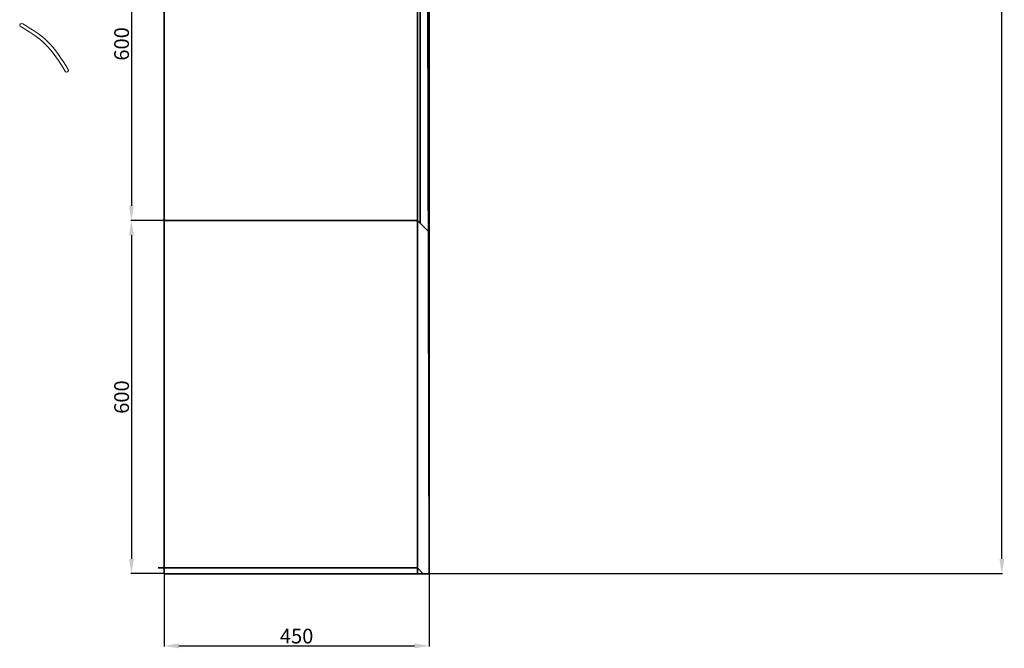
# Model space of a CAD drawing. Units: millimetres. Extents: x 11557 to 15272, y 8572 to 13242.
# Tile 2 of 4: x 13600 to 15272, y 8572 to 9640. Entities that reach past the tile are written whole.
import ezdxf

# ---------------------------------------------------------------- set-up
doc = ezdxf.new("R2010")
doc.units = ezdxf.units.MM
for name, color, linetype, lineweight in [('A-ANNO-DIMS', 2, 'Continuous', 18), ('A-FURN-BASE', 7, 'Continuous', 35), ('A-FURN-HARD', 8, 'Continuous', 18)]:
    doc.layers.add(name, color=color, linetype=linetype, lineweight=lineweight)
doc.styles.get("Standard").update_dxf_attribs({"font": 'arial.ttf'})
doc.dimstyles.new('ISO-25', dxfattribs={"dimtxt": 25, "dimasz": 25, "dimexe": 1.25, "dimexo": 0.625, "dimtad": 1, "dimdec": 1, "dimtxsty": 'Standard', "dimcen": 2.5, "dimadec": 0, "dimazin": 0, "dimtfac": 1, "dimtdec": 1, "dimtmove": 0, "dimatfit": 3, "dimfxl": 1, "dimarcsym": 0})

# ---------------------------------------------------------------- blocks, each defined once
blk = doc.blocks.new('*D1')
at = {"layer": 'A-ANNO-DIMS', "color": 0, "lineweight": -2, "transparency": 16777216}
for p, q in [((13844.6, 9298.9), (13788.4, 9298.9)), ((13789.6, 9273.9), (13789.6, 8723.9)), ((13844.6, 8698.9), (13788.4, 8698.9))]:
    blk.add_line(p, q, dxfattribs=at)
at = {"layer": 'A-ANNO-DIMS', "color": 0, "transparency": 16777216}
for points in [[(13785.5, 9273.9), (13793.8, 9273.9), (13789.6, 9298.9)], [(13785.5, 8723.9), (13793.8, 8723.9), (13789.6, 8698.9)]]:
    blk.add_solid(points, dxfattribs=at)
at = {"layer": 'Defpoints', "color": 0, "transparency": 16777216}
for p in [(13845.2, 9298.9, 720), (13789.6, 8698.9), (13845.2, 8698.9, 720)]:
    blk.add_point(p, dxfattribs=at)
at = {"layer": 'A-ANNO-DIMS', "color": 0, "transparency": 16777216, "insert": (13776.2, 8998.9), "char_height": 25, "attachment_point": 5, "rotation": 90}
blk.add_mtext('600', dxfattribs=at)
blk = doc.blocks.new('*D2')
at = {"layer": 'A-ANNO-DIMS', "color": 0, "lineweight": -2, "transparency": 16777216}
for p, q in [((13844.6, 9898.9), (13788.4, 9898.9)), ((13789.6, 9873.9), (13789.6, 9323.9)), ((13844.6, 9298.9), (13788.4, 9298.9))]:
    blk.add_line(p, q, dxfattribs=at)
at = {"layer": 'A-ANNO-DIMS', "color": 0, "transparency": 16777216}
for points in [[(13785.5, 9873.9), (13793.8, 9873.9), (13789.6, 9898.9)], [(13785.5, 9323.9), (13793.8, 9323.9), (13789.6, 9298.9)]]:
    blk.add_solid(points, dxfattribs=at)
at = {"layer": 'Defpoints', "color": 0, "transparency": 16777216}
for p in [(13845.2, 9898.9, 720), (13789.6, 9298.9), (13845.2, 9298.9, 720)]:
    blk.add_point(p, dxfattribs=at)
at = {"layer": 'A-ANNO-DIMS', "color": 0, "transparency": 16777216, "insert": (13776.2, 9598.9), "char_height": 25, "attachment_point": 5, "rotation": 90}
blk.add_mtext('600', dxfattribs=at)
blk = doc.blocks.new('BASE-CABINET-PULL')
for centre, radius, start, end in [((3, 79.7, -122.8), 3.04, 50.0455, 215.1607), ((79.2, 3.1, -122.8), 3.13, 238.0113, 27.1949)]:
    blk.add_arc(centre, radius, start, end)
for points in [[(77.6, 0.5, -122.8), (66.9, 17.8, -122.8), (47.2, 49.7, -122.8), (15.2, 69.1, -122.8), (0.5, 77.9, -122.8)], [(82, 4.6, -122.8), (71.3, 21.8, -122.8), (51.6, 53.8, -122.8), (19.6, 73.1, -122.8), (5, 82, -122.8)]]:
    blk.add_open_spline(points, degree=3, knots=[0, 0, 0, 0, 59.935873, 110.632609, 110.632609, 110.632609, 110.632609])
blk = doc.blocks.new('*D33')
at = {"layer": 'A-ANNO-DIMS', "color": 0, "lineweight": -2, "transparency": 16777216}
for p, q in [((13845.2, 8698.2), (13845.2, 8575)), ((14295.2, 8698.2), (14295.2, 8575)), ((13870.2, 8576.2), (14270.2, 8576.2))]:
    blk.add_line(p, q, dxfattribs=at)
at = {"layer": 'A-ANNO-DIMS', "color": 0, "transparency": 16777216}
for points in [[(13870.2, 8580.4), (13870.2, 8572), (13845.2, 8576.2)], [(14270.2, 8580.4), (14270.2, 8572), (14295.2, 8576.2)]]:
    blk.add_solid(points, dxfattribs=at)
at = {"layer": 'Defpoints', "color": 0, "transparency": 16777216}
for p in [(13845.2, 8698.9), (14295.2, 8698.9), (14295.2, 8576.2)]:
    blk.add_point(p, dxfattribs=at)
at = {"layer": 'A-ANNO-DIMS', "color": 0, "transparency": 16777216, "insert": (14070.2, 8589.6), "char_height": 25, "attachment_point": 5}
blk.add_mtext('450', dxfattribs=at)
blk = doc.blocks.new('*D35')
at = {"layer": 'A-ANNO-DIMS', "color": 0, "lineweight": -2, "transparency": 16777216}
for p, q in [((15145.9, 11098.9), (15269.1, 11098.9)), ((15267.9, 8723.9), (15267.9, 11073.9)), ((14295.9, 8698.9), (15269.1, 8698.9))]:
    blk.add_line(p, q, dxfattribs=at)
at = {"layer": 'A-ANNO-DIMS', "color": 0, "transparency": 16777216}
for points in [[(15263.7, 11073.9), (15272.1, 11073.9), (15267.9, 11098.9)], [(15263.7, 8723.9), (15272.1, 8723.9), (15267.9, 8698.9)]]:
    blk.add_solid(points, dxfattribs=at)
at = {"layer": 'Defpoints', "color": 0, "transparency": 16777216}
for p in [(15145.2, 11098.9), (15267.9, 11098.9), (14295.2, 8698.9)]:
    blk.add_point(p, dxfattribs=at)
at = {"layer": 'A-ANNO-DIMS', "color": 0, "transparency": 16777216, "insert": (15254.5, 9898.9), "char_height": 25, "attachment_point": 5, "rotation": 90}
blk.add_mtext('2400', dxfattribs=at)

msp = doc.modelspace()

# ---------------------------------------------------------------- linework, layer by layer
at = {"layer": 'A-FURN-BASE'}
for p, q in [((14275.243, 9298.859, 720), (14275.243, 10498.859, 720)), ((14291.462, 10482.64, 136.098), (14295.243, 8708.859, 136.098)), ((14295.243, 9278.848), (14295.243, 10478.859)), ((13845.243, 9298.859, 720), (13845.243, 9898.859, 720)), ((14280.219, 9293.883, 565.291), (14280.219, 9893.883, 565.291)), ((14280.219, 9293.883, 237.922), (14280.219, 9893.883, 237.922)), ((14295.243, 9898.859, 720), (14295.243, 9298.859, 720)), ((13845.243, 8698.859, 720), (13845.243, 9298.859, 720)), ((13845.243, 9298.859, 720), (14275.243, 9298.859, 720)), ((14275.243, 8698.859, 720), (14275.243, 9298.859, 720)), ((14275.243, 9298.859, 720), (14294.025, 9280.077, 136.098)), ((14295.243, 8698.859, 720), (14295.243, 9298.859, 720)), ((14295.243, 8718.859), (14295.243, 9278.848)), ((14295.243, 8998.859, 720), (14294.625, 8998.858, 136.098)), ((14295.243, 8708.859), (14295.243, 8718.859)), ((14275.243, 8708.859, 136.098), (13835.243, 8708.859, 136.098)), ((13845.243, 8698.859), (13845.243, 8698.859, 720)), ((14275.243, 8698.859, 720), (13845.243, 8698.859, 720)), ((14295.243, 8698.859), (13845.243, 8698.859)), ((14295.243, 8698.859, 136.098), (13845.243, 8698.859, 136.098)), ((14295.243, 8698.859, 700), (13845.243, 8698.859, 700)), ((14285.243, 8698.859, 700), (14275.243, 8708.859, 136.098)), ((14275.243, 8698.859, 720), (14275.243, 8698.859, 700)), ((14285.243, 8698.859, 136.098), (14285.243, 8698.859)), ((14295.243, 8698.859), (14295.243, 8708.859)), ((14295.243, 8708.859, 136.098), (14295.243, 8698.859, 136.098)), ((14295.243, 8698.859, 720), (14295.243, 8698.859, 136.098)), ((14295.243, 8698.859, 136.098), (14295.243, 8698.859))]:
    msp.add_line(p, q, dxfattribs=at)

# ---------------------------------------------------------------- block references
at = {"layer": 'A-FURN-HARD'}
msp.add_blockref('BASE-CABINET-PULL', (13600.211, 9551.055), dxfattribs=at)

# ---------------------------------------------------------------- dimensions: what is measured, and where the dimension line sits
at = {"layer": 'A-ANNO-DIMS'}
dim = msp.add_linear_dim(base=(15267.893, 11098.859), p1=(14295.243, 8698.859), p2=(15145.243, 11098.859), angle=90, dimstyle='ISO-25', override={"dimdec": 0, "dimlfac": 1, "dimrnd": 0, "dimzin": 0, "dimdsep": 46, "dimlunit": 2}, dxfattribs=at)
dim.commit()
dim.dimension.update_dxf_attribs({"geometry": '*D35', "text_midpoint": (15254.503, 9898.859)})
for base, p1, p2, picture, middle in [((13789.623, 9298.859, 720), (13845.243, 9898.859, 1440), (13845.243, 9298.859, 1440), '*D2', (13789.623, 9598.859, 720)), ((13789.623, 8698.859, 720), (13845.243, 9298.859, 1440), (13845.243, 8698.859, 1440), '*D1', (13789.623, 8998.859, 720))]:
    dim = msp.add_linear_dim(base=base, p1=p1, p2=p2, angle=90, dimstyle='ISO-25', override={"dimclrd": 0, "dimclre": 0, "dimclrt": 0}, dxfattribs=at)
    dim.commit()
    dim.dimension.update_dxf_attribs({"geometry": picture, "text_midpoint": middle, "dimtype": 160})
dim = msp.add_linear_dim(base=(14295.243, 8576.209), p1=(13845.243, 8698.859), p2=(14295.243, 8698.859), dimstyle='ISO-25', override={"dimdec": 0, "dimlfac": 1, "dimrnd": 0, "dimzin": 0, "dimdsep": 46, "dimlunit": 2}, dxfattribs=at)
dim.commit()
dim.dimension.update_dxf_attribs({"geometry": '*D33', "text_midpoint": (14070.243, 8589.598)})

doc.saveas('drawing.dxf')
